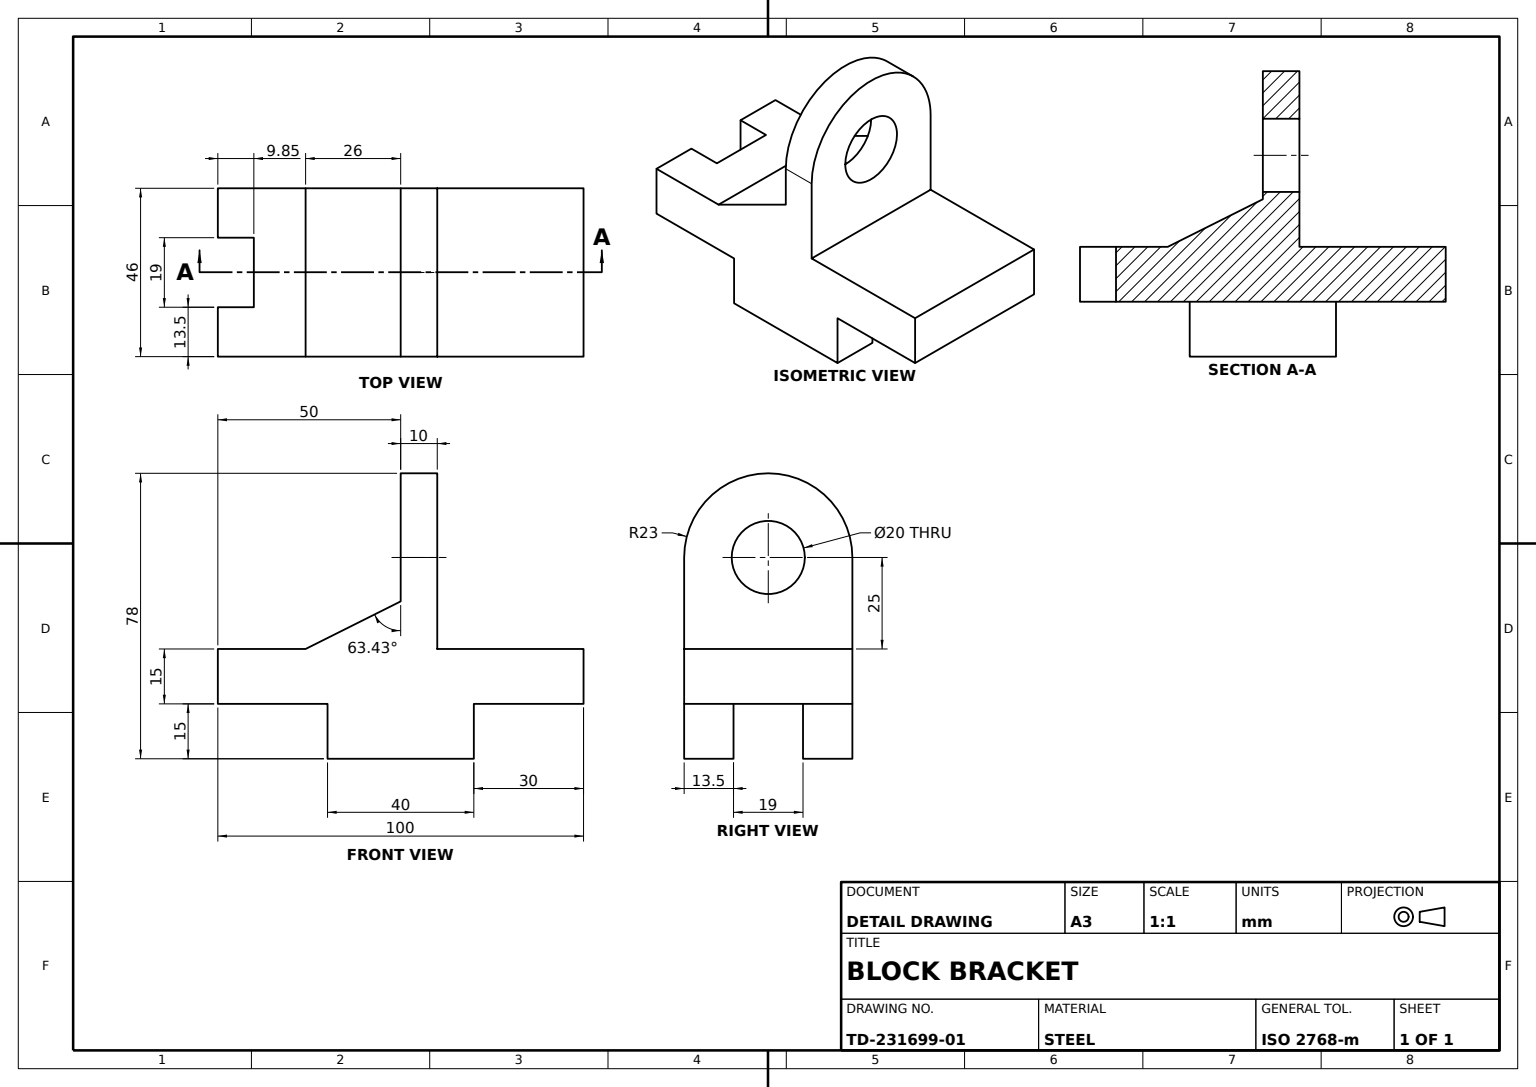
SolidWorks part; units mm, degrees
material "Plain Carbon Steel"
ref_plane "Front Plane" through (0, 0, 0) normal (0, 0, 1) x (1, 0, 0)
ref_plane "Top Plane" through (0, 0, 0) normal (0, 1, 0) x (1, 0, 0)
ref_plane "Right Plane" through (0, 0, 0) normal (1, 0, 0) x (0, 0, -1)
sketch "Base Plate Sketch" plane through (0, 0, 0) normal (0, 1, 0) x (1, 0, 0)
  line L0 (13.5, 0) -> (13.5, 9.8476)
  line L1 (0, 0) -> (13.5, 0)
  line L2 (0, 0) -> (0, 100)
  line L3 (0, 100) -> (46, 100)
  line L4 (46, 0) -> (46, 100)
  line L5 (13.5, 9.8476) -> (32.5, 9.8476)
  line L6 (32.5, 9.8476) -> (32.5, 0)
  line L7 (32.5, 0) -> (46, 0)
  dimension "D1" = 100
  dimension "D2" = 46
  dimension "D3" = 13.5
  dimension "D4" = 19
  dimension "D5" = 13.5
  dimension "D6" = 9.8476
extrude "Base Plate" add sketch "Base Plate Sketch" along normal blind 15
sketch "Side Block A Sketch" plane through (0, 0, 0) normal (1, 0, 0) x (0, 0, -1)
  line L0 (30, 0) -> (70, 0)
  line L1 (0, 0) -> (100, 0) construction
  line L2 (70, 0) -> (70, -15)
  line L3 (70, -15) -> (30, -15)
  line L4 (30, -15) -> (30, 0)
  dimension "D1" = 15
  dimension "D2" = 30
  dimension "D3" = 40
extrude "Side Block A" add sketch "Side Block A Sketch" along normal blind 13.5
ref_plane "Plane2" through (46, 0, 0) normal (1, 0, 0) x (0, 0, -1)
sketch "Side Block B Sketch" plane through (46, 0, 0) normal (1, 0, 0) x (0, 0, -1)
  line L0 (30, 0) -> (70, 0)
  line L1 (30, 0) -> (30, -15) construction
  line L2 (70, -15) -> (70, 0) construction
  line L3 (70, 0) -> (70, -15)
  line L4 (70, -15) -> (30, -15)
  line L5 (30, -15) -> (30, 0)
  dimension "D1" = 30
  dimension "D2" = 30
  dimension "D3" = 40
  dimension "D4" = 15
extrude "Side Block B" add sketch "Side Block B Sketch" against normal blind 13.5
sketch "Upright Web Sketch" plane through (0, 15, 0) normal (0, 1, 0) x (1, 0, 0)
  line L0 (46, 100) -> (46, 60)
  line L1 (46, -7.2287) -> (46, 7.2287) construction
  line L2 (46, 100) -> (0, 100) construction
  line L3 (46, 60) -> (0, 60)
  line L4 (0, 100) -> (0, 0) construction
  line L5 (0, 60) -> (0, 100)
  line L6 (46, 0) -> (46, 24)
  line L7 (32.5, 0) -> (46, 0) construction
  line L8 (46, 24) -> (0, 24)
  line L9 (0, 24) -> (0, 0)
  line L10 (46, 60) -> (46, 50)
  line L11 (46, 50) -> (0, 50)
  line L12 (0, 50) -> (0, 60)
  line L13 (0, 60) -> (0, 50)
  line M7 (0, 100) -> (0, 0)
  line M13 (46, 0) -> (46, 100)
  dimension "D1" = 40
  dimension "D2" = 40
  dimension "D3" = 24
  dimension "D4" = 24
  dimension "D5" = 10
  dimension "D6" = 10
extrude "Upright Web" add sketch "Upright Web Sketch" along normal blind 25 contours L11 L3 M13 M7
ref_plane "Plane4" through (0, 0, -50) normal (0, 0, 1) x (1, 0, 0)
sketch "Lug Ear Sketch" plane through (0, 0, -50) normal (0, 0, 1) x (1, 0, 0)
  line L0 (46, 40) -> (0, 40) construction
  line L1 (13, 40) -> (0, 40)
  line L2 (33, 40) -> (46, 40)
  circle A0 centre (23, 40) radius 23
  circle A1 centre (23, 40) radius 10
  dimension "D1" = 20
  dimension "D2" = 46
extrude "Lug Ear" add sketch "Lug Ear Sketch" against normal blind 10 contours A1 L2 A0 L1
sketch "Lug Hole Sketch" plane through (0, 0, -50) normal (0, 0, 1) x (1, 0, 0)
  line L0 (33, 40) -> (13, 40) construction
  circle A0 centre (23, 40) radius 10
extrude "Lug Hole" cut sketch "Lug Hole Sketch" against normal blind 10
sketch "Gusset Sketch" plane through (46, 0, 0) normal (1, 0, 0) x (0, 0, -1)
  line L0 (50, 15) -> (24, 15)
  line L1 (50, 25.3) -> (50, -25.3) construction
  line L2 (0, 15) -> (50, 15) construction
  line L3 (24, 15) -> (50, 28)
  line L4 (50, 28) -> (50, 15)
  dimension "D1" = 26
  dimension "D2" = 13
extrude "Gusset" add sketch "Gusset Sketch" against normal blind 46
equation "\"13.5.mm\"=23"
